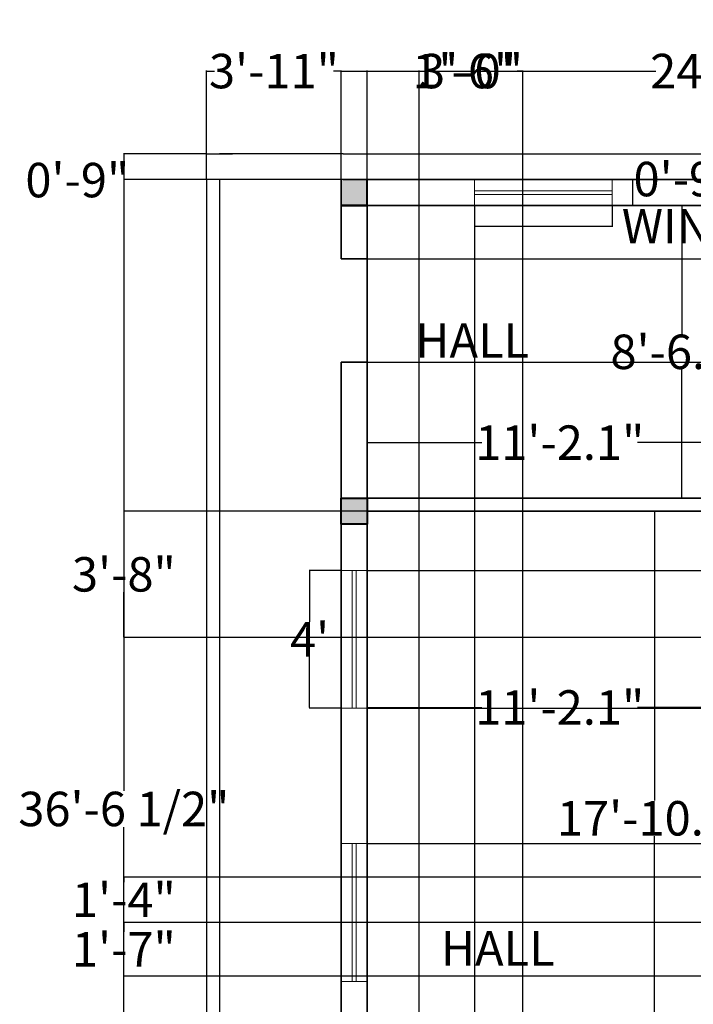
# Model space of a CAD drawing. Units: inches. Extents: x -132 to 363, y -548 to 79.
# Tile 2 of 3: x -107 to 128, y -264 to 79. Entities that reach past the tile are written whole.
import ezdxf

# ---------------------------------------------------------------- set-up
doc = ezdxf.new("R2010")
doc.units = ezdxf.units.IN
doc.header["$MEASUREMENT"] = 0
for name, color, linetype, lineweight in [('A-ANNO-DIMS', 2, 'Continuous', 18), ('A-AREA-IDEN', 7, 'Continuous', 25), ('A-COLS', 7, 'Continuous', 40), ('A-COLS-PATT', 252, 'Continuous', 13), ('A-GLAZ', 4, 'Continuous', 18), ('A-WALL', 7, 'Continuous', 35), ('C-PROP', 8, 'Continuous', 25)]:
    doc.layers.add(name, color=color, linetype=linetype, lineweight=lineweight)
doc.styles.get("Standard").update_dxf_attribs({"font": 'arial.ttf'})
doc.dimstyles.get("Standard").update_dxf_attribs({"dimtxt": 12, "dimasz": 0.18, "dimexe": 0.18, "dimexo": 0.0625, "dimgap": 0.09, "dimtad": 0, "dimtih": 1, "dimtoh": 1, "dimdec": 1, "dimzin": 0, "dimdsep": 46, "dimlunit": 3, "dimtxsty": 'Standard', "dimcen": 0.09, "dimadec": 0, "dimazin": 0, "dimtfac": 1, "dimtdec": 1, "dimtofl": 0, "dimtmove": 0, "dimatfit": 3, "dimfxl": 1, "dimtolj": 1, "dimtzin": 0, "dimarcsym": 0})

# ---------------------------------------------------------------- blocks, each defined once
blk = doc.blocks.new('*D1')
at = {"layer": 'A-ANNO-DIMS', "color": 0, "lineweight": -2, "transparency": 16777216}
for p, q in [((14.42, -87.55), (14.42, -68.07)), ((14.6, -68.25), (54.36, -68.25)), ((148.38, -68.25), (108.61, -68.25)), ((148.56, -87.55), (148.56, -68.07))]:
    blk.add_line(p, q, dxfattribs=at)
at = {"layer": 'A-ANNO-DIMS', "color": 0, "transparency": 16777216}
for points in [[(14.6, -68.22), (14.6, -68.28), (14.42, -68.25)], [(148.38, -68.22), (148.38, -68.28), (148.56, -68.25)]]:
    blk.add_solid(points, dxfattribs=at)
at = {"layer": 'Defpoints', "color": 0, "transparency": 16777216}
for p in [(148.56, -68.25), (14.42, -87.61), (148.56, -87.61)]:
    blk.add_point(p, dxfattribs=at)
at = {"layer": 'A-ANNO-DIMS', "color": 0, "transparency": 16777216, "insert": (81.49, -68.25), "char_height": 12, "attachment_point": 5}
blk.add_mtext('\\A1;11\'-2.1"', dxfattribs=at)
blk = doc.blocks.new('*D2')
at = {"layer": 'A-ANNO-DIMS', "color": 0, "lineweight": -2, "transparency": 16777216}
for p, q in [((148.4, 14.39), (123.86, 14.39)), ((124.04, 14.21), (124.04, -30.39)), ((124.04, -87.43), (124.04, -42.82)), ((148.45, -87.61), (123.86, -87.61))]:
    blk.add_line(p, q, dxfattribs=at)
at = {"layer": 'A-ANNO-DIMS', "color": 0, "transparency": 16777216}
for points in [[(124.01, 14.21), (124.07, 14.21), (124.04, 14.39)], [(124.01, -87.43), (124.07, -87.43), (124.04, -87.61)]]:
    blk.add_solid(points, dxfattribs=at)
at = {"layer": 'Defpoints', "color": 0, "transparency": 16777216}
for p in [(124.04, 14.39), (148.46, 14.39), (148.52, -87.61)]:
    blk.add_point(p, dxfattribs=at)
at = {"layer": 'A-ANNO-DIMS', "color": 0, "transparency": 16777216, "insert": (124.04, -36.61), "char_height": 12, "attachment_point": 5}
blk.add_mtext('\\A1;8\'-6.0"', dxfattribs=at)
blk = doc.blocks.new('*D15')
at = {"layer": 'A-ANNO-DIMS', "color": 0, "lineweight": -2, "transparency": 16777216}
for p, q in [((14.42, -160.68), (14.42, -160.33)), ((14.6, -160.51), (54.34, -160.51)), ((148.34, -160.51), (108.59, -160.51)), ((148.52, -160.68), (148.52, -160.33))]:
    blk.add_line(p, q, dxfattribs=at)
at = {"layer": 'A-ANNO-DIMS', "color": 0, "transparency": 16777216}
for points in [[(14.6, -160.48), (14.6, -160.54), (14.42, -160.51)], [(148.34, -160.48), (148.34, -160.54), (148.52, -160.51)]]:
    blk.add_solid(points, dxfattribs=at)
at = {"layer": 'Defpoints', "color": 0, "transparency": 16777216}
for p in [(14.42, -160.75), (148.52, -160.51), (148.52, -160.75)]:
    blk.add_point(p, dxfattribs=at)
at = {"layer": 'A-ANNO-DIMS', "color": 0, "transparency": 16777216, "insert": (81.47, -160.51), "char_height": 12, "attachment_point": 5}
blk.add_mtext('\\A1;11\'-2.1"', dxfattribs=at)
blk = doc.blocks.new('*D16')
at = {"layer": 'A-ANNO-DIMS', "color": 0, "lineweight": -2, "transparency": 16777216}
for p, q in [((148.45, -92.11), (114.32, -92.11)), ((114.5, -92.29), (114.5, -192.89)), ((114.5, -305.93), (114.5, -205.32)), ((148.45, -306.11), (114.32, -306.11))]:
    blk.add_line(p, q, dxfattribs=at)
at = {"layer": 'A-ANNO-DIMS', "color": 0, "transparency": 16777216}
for points in [[(114.47, -92.29), (114.53, -92.29), (114.5, -92.11)], [(114.47, -305.93), (114.53, -305.93), (114.5, -306.11)]]:
    blk.add_solid(points, dxfattribs=at)
at = {"layer": 'Defpoints', "color": 0, "transparency": 16777216}
for p in [(148.52, -92.11), (114.5, -306.11), (148.52, -306.11)]:
    blk.add_point(p, dxfattribs=at)
at = {"layer": 'A-ANNO-DIMS', "color": 0, "transparency": 16777216, "insert": (114.5, -199.11), "char_height": 12, "attachment_point": 5}
blk.add_mtext('\\A1;17\'-10.0"', dxfattribs=at)
blk = doc.blocks.new('*D17')
at = {"layer": 'A-ANNO-DIMS', "color": 0, "lineweight": -2, "transparency": 16777216}
for p, q in [((5.35, -112.75), (-5.8, -112.75)), ((-5.62, -112.93), (-5.62, -130.66)), ((-5.62, -160.57), (-5.62, -142.84)), ((5.35, -160.75), (-5.8, -160.75))]:
    blk.add_line(p, q, dxfattribs=at)
at = {"layer": 'A-ANNO-DIMS', "color": 0, "transparency": 16777216}
for points in [[(-5.65, -112.93), (-5.59, -112.93), (-5.62, -112.75)], [(-5.65, -160.57), (-5.59, -160.57), (-5.62, -160.75)]]:
    blk.add_solid(points, dxfattribs=at)
at = {"layer": 'Defpoints', "color": 0, "transparency": 16777216}
for p in [(-5.62, -112.75), (5.42, -112.75), (5.42, -160.75)]:
    blk.add_point(p, dxfattribs=at)
at = {"layer": 'A-ANNO-DIMS', "color": 0, "transparency": 16777216, "insert": (-5.62, -136.75), "char_height": 12, "attachment_point": 5}
blk.add_mtext("\\A1;4'", dxfattribs=at)
blk = doc.blocks.new('WIN-48IN')
for p, q in [((48, 9), (0, 9)), ((0, 9), (0, 0)), ((48, 0), (48, 9)), ((0, 5.12), (48, 5.12)), ((48, 5.12), (0, 5.12)), ((0, 3.8), (48, 3.8)), ((0, 0), (48, 0))]:
    blk.add_line(p, q)
blk = doc.blocks.new('*D21')
at = {"layer": 'A-ANNO-DIMS', "color": 0, "lineweight": -2, "transparency": 16777216}
for p, q in [((51.75, 14.33), (51.75, 7.01)), ((99.75, 14.33), (99.75, 7.01)), ((51.93, 7.19), (99.57, 7.19)), ((99.75, 7.19), (99.93, 7.19))]:
    blk.add_line(p, q, dxfattribs=at)
at = {"layer": 'A-ANNO-DIMS', "color": 0, "transparency": 16777216}
for points in [[(51.93, 7.22), (51.93, 7.16), (51.75, 7.19)], [(99.57, 7.22), (99.57, 7.16), (99.75, 7.19)]]:
    blk.add_solid(points, dxfattribs=at)
at = {"layer": 'Defpoints', "color": 0, "transparency": 16777216}
for p in [(51.75, 14.39), (99.75, 14.39), (99.75, 7.19)]:
    blk.add_point(p, dxfattribs=at)
at = {"layer": 'A-ANNO-DIMS', "color": 0, "transparency": 16777216, "insert": (175.94, 7.19), "char_height": 12, "attachment_point": 5}
blk.add_mtext('\\A1;WINDOW 4\'-0" TYP.', dxfattribs=at)
blk = doc.blocks.new('*D22')
at = {"layer": 'A-ANNO-DIMS', "color": 0, "lineweight": -2, "transparency": 16777216}
for p, q in [((99.81, 23.39), (107.13, 23.39)), ((106.95, 23.39), (106.95, 23.57)), ((106.95, 23.57), (107.13, 23.57)), ((106.95, 14.57), (106.95, 23.21)), ((99.81, 14.39), (107.13, 14.39))]:
    blk.add_line(p, q, dxfattribs=at)
at = {"layer": 'A-ANNO-DIMS', "color": 0, "transparency": 16777216}
for points in [[(106.92, 23.21), (106.98, 23.21), (106.95, 23.39)], [(106.92, 14.57), (106.98, 14.57), (106.95, 14.39)]]:
    blk.add_solid(points, dxfattribs=at)
at = {"layer": 'Defpoints', "color": 0, "transparency": 16777216}
for p in [(99.75, 23.39), (106.95, 23.39), (99.75, 14.39)]:
    blk.add_point(p, dxfattribs=at)
at = {"layer": 'A-ANNO-DIMS', "color": 0, "transparency": 16777216, "insert": (143.79, 23.57), "char_height": 12, "attachment_point": 5}
blk.add_mtext('\\A1;0\'-9" TYP.', dxfattribs=at)
blk = doc.blocks.new('*D27')
at = {"layer": 'A-ANNO-DIMS', "color": 0, "lineweight": -2, "transparency": 16777216}
for p, q in [((5.42, 23.45), (5.42, 61.37)), ((5.6, 61.19), (114.93, 61.19)), ((293.84, 61.19), (184.5, 61.19)), ((294.02, 23.45), (294.02, 61.37))]:
    blk.add_line(p, q, dxfattribs=at)
at = {"layer": 'A-ANNO-DIMS', "color": 0, "transparency": 16777216}
for points in [[(5.6, 61.22), (5.6, 61.16), (5.42, 61.19)], [(293.84, 61.22), (293.84, 61.16), (294.02, 61.19)]]:
    blk.add_solid(points, dxfattribs=at)
at = {"layer": 'Defpoints', "color": 0, "transparency": 16777216}
for p in [(294.02, 61.19), (5.42, 23.39), (294.02, 23.39)]:
    blk.add_point(p, dxfattribs=at)
at = {"layer": 'A-ANNO-DIMS', "color": 0, "transparency": 16777216, "insert": (149.72, 61.19), "char_height": 12, "attachment_point": 5}
blk.add_mtext('\\A1;24\'-0 1/2"', dxfattribs=at)
blk = doc.blocks.new('*D28')
at = {"layer": 'A-ANNO-DIMS', "color": 0, "lineweight": -2, "transparency": 16777216}
for p, q in [((-41.48, 32.45), (-41.48, 61.37)), ((-41.3, 61.19), (-38.73, 61.19)), ((5.24, 61.19), (2.66, 61.19)), ((5.42, 23.45), (5.42, 61.37))]:
    blk.add_line(p, q, dxfattribs=at)
at = {"layer": 'A-ANNO-DIMS', "color": 0, "transparency": 16777216}
for points in [[(-41.3, 61.22), (-41.3, 61.16), (-41.48, 61.19)], [(5.24, 61.22), (5.24, 61.16), (5.42, 61.19)]]:
    blk.add_solid(points, dxfattribs=at)
at = {"layer": 'Defpoints', "color": 0, "transparency": 16777216}
for p in [(5.42, 61.19), (-41.48, 32.39), (5.42, 23.39)]:
    blk.add_point(p, dxfattribs=at)
at = {"layer": 'A-ANNO-DIMS', "color": 0, "transparency": 16777216, "insert": (-18.03, 61.19), "char_height": 12, "attachment_point": 5}
blk.add_mtext('\\A1;3\'-11"', dxfattribs=at)
blk = doc.blocks.new('*D29')
at = {"layer": 'A-ANNO-DIMS', "color": 0, "lineweight": -2, "transparency": 16777216}
for p, q in [((14.42, 14.33), (14.42, -530.59)), ((51.75, 14.33), (51.75, -530.59)), ((14.6, -530.41), (51.57, -530.41)), ((51.75, -530.41), (51.93, -530.41))]:
    blk.add_line(p, q, dxfattribs=at)
at = {"layer": 'A-ANNO-DIMS', "color": 0, "transparency": 16777216}
for points in [[(14.6, -530.38), (14.6, -530.44), (14.42, -530.41)], [(51.57, -530.38), (51.57, -530.44), (51.75, -530.41)]]:
    blk.add_solid(points, dxfattribs=at)
at = {"layer": 'Defpoints', "color": 0, "transparency": 16777216}
for p in [(14.42, 14.39), (51.75, 14.39), (51.75, -530.41)]:
    blk.add_point(p, dxfattribs=at)
at = {"layer": 'A-ANNO-DIMS', "color": 0, "transparency": 16777216, "insert": (81.94, -530.41), "char_height": 12, "attachment_point": 5}
blk.add_mtext('\\A1;3\'-1 1/2"', dxfattribs=at)
blk = doc.blocks.new('*D31')
at = {"layer": 'A-ANNO-DIMS', "color": 0, "lineweight": -2, "transparency": 16777216}
for p, q in [((14.48, 14.39), (332, 14.39)), ((331.82, 14.21), (331.82, 11.36)), ((331.82, -4.08), (331.82, -1.23)), ((14.48, -4.26), (332, -4.26))]:
    blk.add_line(p, q, dxfattribs=at)
at = {"layer": 'A-ANNO-DIMS', "color": 0, "transparency": 16777216}
for points in [[(331.79, 14.21), (331.85, 14.21), (331.82, 14.39)], [(331.79, -4.08), (331.85, -4.08), (331.82, -4.26)]]:
    blk.add_solid(points, dxfattribs=at)
at = {"layer": 'Defpoints', "color": 0, "transparency": 16777216}
for p in [(14.42, 14.39), (14.42, -4.26), (331.82, -4.26)]:
    blk.add_point(p, dxfattribs=at)
at = {"layer": 'A-ANNO-DIMS', "color": 0, "transparency": 16777216, "insert": (331.82, 5.07), "char_height": 12, "attachment_point": 5}
blk.add_mtext('\\A1;1\'-6 1/2"', dxfattribs=at)
blk = doc.blocks.new('*D32')
at = {"layer": 'A-ANNO-DIMS', "color": 0, "lineweight": -2, "transparency": 16777216}
for p, q in [((14.48, -4.26), (332, -4.26)), ((331.82, -4.44), (331.82, -16.04)), ((331.82, -40.08), (331.82, -28.48)), ((14.48, -40.26), (332, -40.26))]:
    blk.add_line(p, q, dxfattribs=at)
at = {"layer": 'A-ANNO-DIMS', "color": 0, "transparency": 16777216}
for points in [[(331.79, -4.44), (331.85, -4.44), (331.82, -4.26)], [(331.79, -40.08), (331.85, -40.08), (331.82, -40.26)]]:
    blk.add_solid(points, dxfattribs=at)
at = {"layer": 'Defpoints', "color": 0, "transparency": 16777216}
for p in [(14.42, -4.26), (14.42, -40.26), (331.82, -40.26)]:
    blk.add_point(p, dxfattribs=at)
at = {"layer": 'A-ANNO-DIMS', "color": 0, "transparency": 16777216, "insert": (331.82, -22.26), "char_height": 12, "attachment_point": 5}
blk.add_mtext('\\A1;3\'-0"', dxfattribs=at)
blk = doc.blocks.new('*D33')
at = {"layer": 'A-ANNO-DIMS', "color": 0, "lineweight": -2, "transparency": 16777216}
for p, q in [((14.48, -92.11), (332, -92.11)), ((331.82, -92.29), (331.82, -96.13)), ((331.82, -112.57), (331.82, -108.72)), ((14.48, -112.75), (332, -112.75))]:
    blk.add_line(p, q, dxfattribs=at)
at = {"layer": 'A-ANNO-DIMS', "color": 0, "transparency": 16777216}
for points in [[(331.79, -92.29), (331.85, -92.29), (331.82, -92.11)], [(331.79, -112.57), (331.85, -112.57), (331.82, -112.75)]]:
    blk.add_solid(points, dxfattribs=at)
at = {"layer": 'Defpoints', "color": 0, "transparency": 16777216}
for p in [(14.42, -92.11), (14.42, -112.75), (331.82, -112.75)]:
    blk.add_point(p, dxfattribs=at)
at = {"layer": 'A-ANNO-DIMS', "color": 0, "transparency": 16777216, "insert": (331.82, -102.43), "char_height": 12, "attachment_point": 5}
blk.add_mtext('\\A1;1\'-8 1/2"', dxfattribs=at)
blk = doc.blocks.new('*D34')
at = {"layer": 'A-ANNO-DIMS', "color": 0, "lineweight": -2, "transparency": 16777216}
for p, q in [((14.48, -160.75), (332, -160.75)), ((331.82, -160.93), (331.82, -178.11)), ((331.82, -207.73), (331.82, -190.55)), ((14.48, -207.91), (332, -207.91))]:
    blk.add_line(p, q, dxfattribs=at)
at = {"layer": 'A-ANNO-DIMS', "color": 0, "transparency": 16777216}
for points in [[(331.79, -160.93), (331.85, -160.93), (331.82, -160.75)], [(331.79, -207.73), (331.85, -207.73), (331.82, -207.91)]]:
    blk.add_solid(points, dxfattribs=at)
at = {"layer": 'Defpoints', "color": 0, "transparency": 16777216}
for p in [(14.42, -160.75), (14.42, -207.91), (331.82, -207.91)]:
    blk.add_point(p, dxfattribs=at)
at = {"layer": 'A-ANNO-DIMS', "color": 0, "transparency": 16777216, "insert": (331.82, -184.33), "char_height": 12, "attachment_point": 5}
blk.add_mtext('\\A1;3\'-11"', dxfattribs=at)
blk = doc.blocks.new('*D35')
at = {"layer": 'A-ANNO-DIMS', "color": 0, "lineweight": -2, "transparency": 16777216}
for p, q in [((284.95, -92.11), (-70.46, -92.11)), ((-70.28, -92.29), (-70.28, -107.91)), ((-70.28, -135.97), (-70.28, -120.35)), ((284.95, -136.15), (-70.46, -136.15))]:
    blk.add_line(p, q, dxfattribs=at)
at = {"layer": 'A-ANNO-DIMS', "color": 0, "transparency": 16777216}
for points in [[(-70.31, -92.29), (-70.25, -92.29), (-70.28, -92.11)], [(-70.31, -135.97), (-70.25, -135.97), (-70.28, -136.15)]]:
    blk.add_solid(points, dxfattribs=at)
at = {"layer": 'Defpoints', "color": 0, "transparency": 16777216}
for p in [(285.02, -92.11), (-70.28, -136.15), (285.02, -136.15)]:
    blk.add_point(p, dxfattribs=at)
at = {"layer": 'A-ANNO-DIMS', "color": 0, "transparency": 16777216, "insert": (-70.28, -114.13), "char_height": 12, "attachment_point": 5}
blk.add_mtext('\\A1;3\'-8"', dxfattribs=at)
blk = doc.blocks.new('*D39')
at = {"layer": 'A-ANNO-DIMS', "color": 0, "lineweight": -2, "transparency": 16777216}
for p, q in [((32.59, -306.05), (32.59, 61.37)), ((32.77, 61.19), (34.56, 61.19)), ((68.41, 61.19), (66.63, 61.19)), ((68.59, -306.05), (68.59, 61.37))]:
    blk.add_line(p, q, dxfattribs=at)
at = {"layer": 'A-ANNO-DIMS', "color": 0, "transparency": 16777216}
for points in [[(32.77, 61.22), (32.77, 61.16), (32.59, 61.19)], [(68.41, 61.22), (68.41, 61.16), (68.59, 61.19)]]:
    blk.add_solid(points, dxfattribs=at)
at = {"layer": 'Defpoints', "color": 0, "transparency": 16777216}
for p in [(68.59, 61.19), (32.59, -306.11), (68.59, -306.11)]:
    blk.add_point(p, dxfattribs=at)
at = {"layer": 'A-ANNO-DIMS', "color": 0, "transparency": 16777216, "insert": (50.59, 61.19), "char_height": 12, "attachment_point": 5}
blk.add_mtext('\\A1;3\'-0"', dxfattribs=at)
blk = doc.blocks.new('*D40')
at = {"layer": 'A-ANNO-DIMS', "color": 0, "lineweight": -2, "transparency": 16777216}
for p, q in [((14.42, -306.05), (14.42, 61.37)), ((14.6, 61.19), (32.41, 61.19)), ((32.59, -306.05), (32.59, 61.37)), ((32.59, 61.19), (32.77, 61.19))]:
    blk.add_line(p, q, dxfattribs=at)
at = {"layer": 'A-ANNO-DIMS', "color": 0, "transparency": 16777216}
for points in [[(14.6, 61.22), (14.6, 61.16), (14.42, 61.19)], [(32.41, 61.22), (32.41, 61.16), (32.59, 61.19)]]:
    blk.add_solid(points, dxfattribs=at)
at = {"layer": 'Defpoints', "color": 0, "transparency": 16777216}
for p in [(32.59, 61.19), (14.42, -306.11), (32.59, -306.11)]:
    blk.add_point(p, dxfattribs=at)
at = {"layer": 'A-ANNO-DIMS', "color": 0, "transparency": 16777216, "insert": (48.25, 61.19), "char_height": 12, "attachment_point": 5}
blk.add_mtext('\\A1;1\'-6"', dxfattribs=at)
blk = doc.blocks.new('*D46')
at = {"layer": 'A-ANNO-DIMS', "color": 0, "lineweight": -2, "transparency": 16777216}
for p, q in [((208.45, -235.36), (-70.46, -235.36)), ((-70.28, -235.54), (-70.28, -238.62)), ((-70.28, -253.94), (-70.28, -250.85)), ((208.45, -254.12), (-70.46, -254.12))]:
    blk.add_line(p, q, dxfattribs=at)
at = {"layer": 'A-ANNO-DIMS', "color": 0, "transparency": 16777216}
for points in [[(-70.31, -235.54), (-70.25, -235.54), (-70.28, -235.36)], [(-70.31, -253.94), (-70.25, -253.94), (-70.28, -254.12)]]:
    blk.add_solid(points, dxfattribs=at)
at = {"layer": 'Defpoints', "color": 0, "transparency": 16777216}
for p in [(208.52, -235.36), (-70.28, -254.12), (208.52, -254.12)]:
    blk.add_point(p, dxfattribs=at)
at = {"layer": 'A-ANNO-DIMS', "color": 0, "transparency": 16777216, "insert": (-70.28, -244.74), "char_height": 12, "attachment_point": 5}
blk.add_mtext('\\A1;1\'-7"', dxfattribs=at)
blk = doc.blocks.new('*D50')
at = {"layer": 'A-ANNO-DIMS', "color": 0, "lineweight": -2, "transparency": 16777216}
for p, q in [((208.45, -219.61), (-70.46, -219.61)), ((-70.28, -219.79), (-70.28, -221.37)), ((208.45, -235.36), (-70.46, -235.36)), ((-70.28, -235.18), (-70.28, -233.6))]:
    blk.add_line(p, q, dxfattribs=at)
at = {"layer": 'A-ANNO-DIMS', "color": 0, "transparency": 16777216}
for points in [[(-70.31, -219.79), (-70.25, -219.79), (-70.28, -219.61)], [(-70.31, -235.18), (-70.25, -235.18), (-70.28, -235.36)]]:
    blk.add_solid(points, dxfattribs=at)
at = {"layer": 'Defpoints', "color": 0, "transparency": 16777216}
for p in [(208.52, -219.61), (-70.28, -235.36), (208.52, -235.36)]:
    blk.add_point(p, dxfattribs=at)
at = {"layer": 'A-ANNO-DIMS', "color": 0, "transparency": 16777216, "insert": (-70.28, -227.48), "char_height": 12, "attachment_point": 5}
blk.add_mtext('\\A1;1\'-4"', dxfattribs=at)
blk = doc.blocks.new('*D53')
at = {"layer": 'A-ANNO-DIMS', "color": 0, "lineweight": -2, "transparency": 16777216}
for p, q in [((5.35, 23.39), (-70.46, 23.39)), ((-70.28, 23.21), (-70.28, -189.56)), ((-70.28, -414.93), (-70.28, -202.16)), ((91.45, -415.11), (-70.46, -415.11))]:
    blk.add_line(p, q, dxfattribs=at)
at = {"layer": 'A-ANNO-DIMS', "color": 0, "transparency": 16777216}
for points in [[(-70.31, 23.21), (-70.25, 23.21), (-70.28, 23.39)], [(-70.31, -414.93), (-70.25, -414.93), (-70.28, -415.11)]]:
    blk.add_solid(points, dxfattribs=at)
at = {"layer": 'Defpoints', "color": 0, "transparency": 16777216}
for p in [(5.42, 23.39), (-70.28, -415.11), (91.52, -415.11)]:
    blk.add_point(p, dxfattribs=at)
at = {"layer": 'A-ANNO-DIMS', "color": 0, "transparency": 16777216, "insert": (-70.28, -195.86), "char_height": 12, "attachment_point": 5}
blk.add_mtext('\\A1;36\'-6 1/2"', dxfattribs=at)
blk = doc.blocks.new('*D54')
at = {"layer": 'A-ANNO-DIMS', "color": 0, "lineweight": -2, "transparency": 16777216}
for p, q in [((-41.55, 32.39), (-70.46, 32.39)), ((-70.28, 32.21), (-70.28, 23.57)), ((-37.05, 23.39), (-70.46, 23.39)), ((-70.28, 23.21), (-70.46, 23.21)), ((-70.28, 23.39), (-70.28, 23.21))]:
    blk.add_line(p, q, dxfattribs=at)
at = {"layer": 'A-ANNO-DIMS', "color": 0, "transparency": 16777216}
for points in [[(-70.31, 32.21), (-70.25, 32.21), (-70.28, 32.39)], [(-70.31, 23.57), (-70.25, 23.57), (-70.28, 23.39)]]:
    blk.add_solid(points, dxfattribs=at)
at = {"layer": 'Defpoints', "color": 0, "transparency": 16777216}
for p in [(-41.48, 32.39), (-70.28, 23.39), (-36.98, 23.39)]:
    blk.add_point(p, dxfattribs=at)
at = {"layer": 'A-ANNO-DIMS', "color": 0, "transparency": 16777216, "insert": (-86.5, 23.21), "char_height": 12, "attachment_point": 5}
blk.add_mtext('\\A1;0\'-9"', dxfattribs=at)

msp = doc.modelspace()

# ---------------------------------------------------------------- hatches: boundary and pattern name
at = {"layer": 'A-COLS-PATT'}
h = msp.add_hatch(color=256, dxfattribs=at)
h.dxf.hatch_style = 1
h.paths.add_polyline_path([(14.42, 23.39), (6.02, 23.39), (5.42, 23.39), (5.42, 14.39), (14.42, 14.39)])
h.paths.add_polyline_path([(14.42, -87.61), (5.42, -87.61), (5.42, -96.61), (14.42, -96.61)])
h.paths.add_polyline_path([(153.02, -87.61), (148.56, -87.61), (148.56, -96.61), (153.02, -96.61)])
h.paths.add_polyline_path([(157.56, -87.61), (153.02, -87.61), (153.02, -92.11), (157.56, -92.11)])
h.paths.add_polyline_path([(157.56, -92.11), (153.02, -92.11), (153.02, -96.61), (157.56, -96.61)])
h.paths.add_polyline_path([(294.02, -87.49), (285.02, -87.49), (285.02, -96.49), (294.02, -96.49)])
h.paths.add_polyline_path([(294.02, -215.01), (285.02, -215.01), (285.02, -224.01), (294.02, -224.01)])
h.paths.add_polyline_path([(294.02, -267.43), (285.02, -267.43), (285.02, -277.01), (294.02, -277.01)])
h.paths.add_polyline_path([(294.02, -406.11), (285.02, -406.11), (285.02, -415.11), (294.02, -415.11)])
h.paths.add_polyline_path([(161.71, -406.11), (148.52, -406.11), (148.52, -415.11), (161.71, -415.11)])
h.paths.add_polyline_path([(157.51, -267.61), (148.52, -267.61), (148.52, -276.61), (157.51, -276.61)])
h.paths.add_polyline_path([(14.42, -268.43), (5.42, -268.43), (5.42, -277.43), (14.42, -277.43)])

# ---------------------------------------------------------------- linework, layer by layer
at = {"layer": 'A-COLS'}
for p, q in [((14.42, 14.39), (14.42, 23.39)), ((14.42, 14.39), (5.42, 14.39)), ((5.42, 14.39), (14.42, 14.39))]:
    msp.add_line(p, q, dxfattribs=at)
msp.add_lwpolyline([(5.42, -87.61), (14.42, -87.61), (14.42, -96.61), (5.42, -96.61)], close=True, dxfattribs=at)
at = {"layer": 'A-WALL'}
for p, q in [((5.42, 23.39), (5.42, -4.26)), ((6.02, 23.39), (294.02, 23.39)), ((14.42, 14.39), (285.02, 14.39)), ((14.42, 14.39), (14.42, -4.26)), ((14.42, -4.26), (5.42, -4.26)), ((5.42, -40.26), (14.42, -40.26)), ((5.42, -40.26), (5.42, -315.11)), ((14.42, -40.26), (14.42, -306.11)), ((14.42, -87.61), (148.52, -87.61)), ((14.42, -92.11), (148.52, -92.11))]:
    msp.add_line(p, q, dxfattribs=at)
at = {"layer": 'C-PROP'}
for p, q in [((-41.48, 23.39), (-41.48, 32.39)), ((-41.48, 32.39), (-32.48, 32.39)), ((6.02, 32.39), (-36.98, 32.39)), ((6.02, 32.39), (294.02, 32.39)), ((-41.48, 23.39), (-41.48, -501.61)), ((6.02, 23.39), (-36.98, 23.39)), ((-36.98, 23.39), (-36.98, -501.61))]:
    msp.add_line(p, q, dxfattribs=at)

# ---------------------------------------------------------------- block references
at = {"layer": 'A-GLAZ'}
msp.add_blockref('WIN-48IN', (51.75, 14.39), dxfattribs=at)
at = {"layer": 'A-GLAZ', "rotation": 269.9999999999999}
for p in [(5.42, -112.75), (5.42, -207.91)]:
    msp.add_blockref('WIN-48IN', p, dxfattribs=at)

# ---------------------------------------------------------------- texts
at = {"layer": 'A-AREA-IDEN'}
for p in [(31.18, -38.69), (40.06, -250.42)]:
    msp.add_text('HALL', height=12, dxfattribs=at).set_placement(p)

# ---------------------------------------------------------------- dimensions: what is measured, and where the dimension line sits
at = {"layer": 'A-ANNO-DIMS'}
for base, p1, p2, override, picture, middle in [((294.02, 61.19), (5.42, 23.39), (294.02, 23.39), {"dimdec": 1, "dimlfac": 1, "dimrnd": 0, "dimzin": 1, "dimdsep": 46, "dimlunit": 4, "dimfrac": 2}, '*D27', (149.72, 61.19)), ((5.42, 61.19), (-41.48, 32.39), (5.42, 23.39), {"dimdec": 1, "dimlfac": 1, "dimrnd": 0, "dimzin": 1, "dimdsep": 46, "dimlunit": 4, "dimfrac": 2}, '*D28', (-18.03, 61.19)), ((32.59, 61.19), (14.42, -306.11), (32.59, -306.11), {"dimdec": 1, "dimlfac": 1, "dimrnd": 0, "dimzin": 1, "dimdsep": 46, "dimlunit": 4, "dimfrac": 2}, '*D40', (48.25, 61.19)), ((68.59, 61.19), (32.59, -306.11), (68.59, -306.11), {"dimdec": 1, "dimlfac": 1, "dimrnd": 0, "dimzin": 1, "dimdsep": 46, "dimlunit": 4, "dimfrac": 2}, '*D39', (50.59, 61.19)), ((51.75, -530.41), (14.42, 14.39), (51.75, 14.39), {"dimdec": 1, "dimlfac": 1, "dimrnd": 0, "dimzin": 1, "dimdsep": 46, "dimlunit": 4, "dimfrac": 2}, '*D29', (81.94, -530.41)), ((148.56, -68.25), (14.42, -87.61), (148.56, -87.61), {"dimclrd": 0, "dimclre": 0, "dimclrt": 0}, '*D1', (81.49, -68.25)), ((148.52, -160.51), (14.42, -160.75), (148.52, -160.75), {"dimclrd": 0, "dimclre": 0, "dimclrt": 0}, '*D15', (81.47, -160.51))]:
    dim = msp.add_linear_dim(base=base, p1=p1, p2=p2, dimstyle='Standard', override=override, dxfattribs=at)
    dim.commit()
    dim.dimension.update_dxf_attribs({"geometry": picture, "text_midpoint": middle})
dim = msp.add_linear_dim(base=(106.95, 23.39), p1=(99.75, 14.39), p2=(99.75, 23.39), angle=90, text='<> TYP.', dimstyle='Standard', override={"dimdec": 1, "dimlfac": 1, "dimrnd": 0, "dimzin": 1, "dimdsep": 46, "dimlunit": 4, "dimfrac": 2}, dxfattribs=at)
dim.commit()
dim.dimension.update_dxf_attribs({"geometry": '*D22', "text_midpoint": (143.79, 23.57)})
dim = msp.add_linear_dim(base=(99.75, 7.19), p1=(51.75, 14.39), p2=(99.75, 14.39), text='WINDOW <> TYP.', dimstyle='Standard', override={"dimdec": 1, "dimlfac": 1, "dimrnd": 0, "dimzin": 1, "dimdsep": 46, "dimlunit": 4, "dimfrac": 2}, dxfattribs=at)
dim.commit()
dim.dimension.update_dxf_attribs({"geometry": '*D21', "text_midpoint": (175.94, 7.19)})
for base, p1, p2, override, picture, middle in [((-70.28, 23.39), (-41.48, 32.39), (-36.98, 23.39), {"dimdec": 1, "dimlfac": 1, "dimrnd": 0, "dimzin": 1, "dimdsep": 46, "dimlunit": 4, "dimfrac": 2}, '*D54', (-86.5, 23.21)), ((-70.28, -415.11), (5.42, 23.39), (91.52, -415.11), {"dimdec": 1, "dimlfac": 1, "dimrnd": 0, "dimzin": 1, "dimdsep": 46, "dimlunit": 4, "dimfrac": 2}, '*D53', (-70.28, -195.86)), ((331.8158, -4.2561), (14.4158, 14.392), (14.4158, -4.2561), {"dimdec": 1, "dimlfac": 1, "dimrnd": 0, "dimzin": 1, "dimdsep": 46, "dimlunit": 4, "dimfrac": 2}, '*D31', (331.8158, 5.068)), ((124.04, 14.39), (148.52, -87.61), (148.46, 14.39), {"dimclrd": 0, "dimclre": 0, "dimclrt": 0}, '*D2', (124.04, -36.61)), ((331.82, -40.26), (14.42, -4.26), (14.42, -40.26), {"dimdec": 1, "dimlfac": 1, "dimrnd": 0, "dimzin": 1, "dimdsep": 46, "dimlunit": 4, "dimfrac": 2}, '*D32', (331.82, -22.26)), ((331.82, -112.75), (14.42, -92.11), (14.42, -112.75), {"dimdec": 1, "dimlfac": 1, "dimrnd": 0, "dimzin": 1, "dimdsep": 46, "dimlunit": 4, "dimfrac": 2}, '*D33', (331.82, -102.43)), ((-70.28, -136.15), (285.02, -92.11), (285.02, -136.15), {"dimdec": 1, "dimlfac": 1, "dimrnd": 0, "dimzin": 1, "dimdsep": 46, "dimlunit": 4, "dimfrac": 2}, '*D35', (-70.28, -114.13)), ((114.5, -306.11), (148.52, -92.11), (148.52, -306.11), {"dimclrd": 0, "dimclre": 0, "dimclrt": 0}, '*D16', (114.5, -199.11)), ((-5.62, -112.75), (5.42, -160.75), (5.42, -112.75), {"dimclrd": 0, "dimclre": 0, "dimclrt": 0}, '*D17', (-5.62, -136.75)), ((331.82, -207.91), (14.42, -160.75), (14.42, -207.91), {"dimdec": 1, "dimlfac": 1, "dimrnd": 0, "dimzin": 1, "dimdsep": 46, "dimlunit": 4, "dimfrac": 2}, '*D34', (331.82, -184.33)), ((-70.2842, -235.3581), (208.5158, -219.608), (208.5158, -235.3581), {"dimdec": 1, "dimlfac": 1, "dimrnd": 0, "dimzin": 1, "dimdsep": 46, "dimlunit": 4, "dimfrac": 2}, '*D50', (-70.2842, -227.483)), ((-70.28, -254.12), (208.52, -235.36), (208.52, -254.12), {"dimdec": 1, "dimlfac": 1, "dimrnd": 0, "dimzin": 1, "dimdsep": 46, "dimlunit": 4, "dimfrac": 2}, '*D46', (-70.28, -244.74))]:
    dim = msp.add_linear_dim(base=base, p1=p1, p2=p2, angle=90, dimstyle='Standard', override=override, dxfattribs=at)
    dim.commit()
    dim.dimension.update_dxf_attribs({"geometry": picture, "text_midpoint": middle})

doc.saveas('drawing.dxf')
